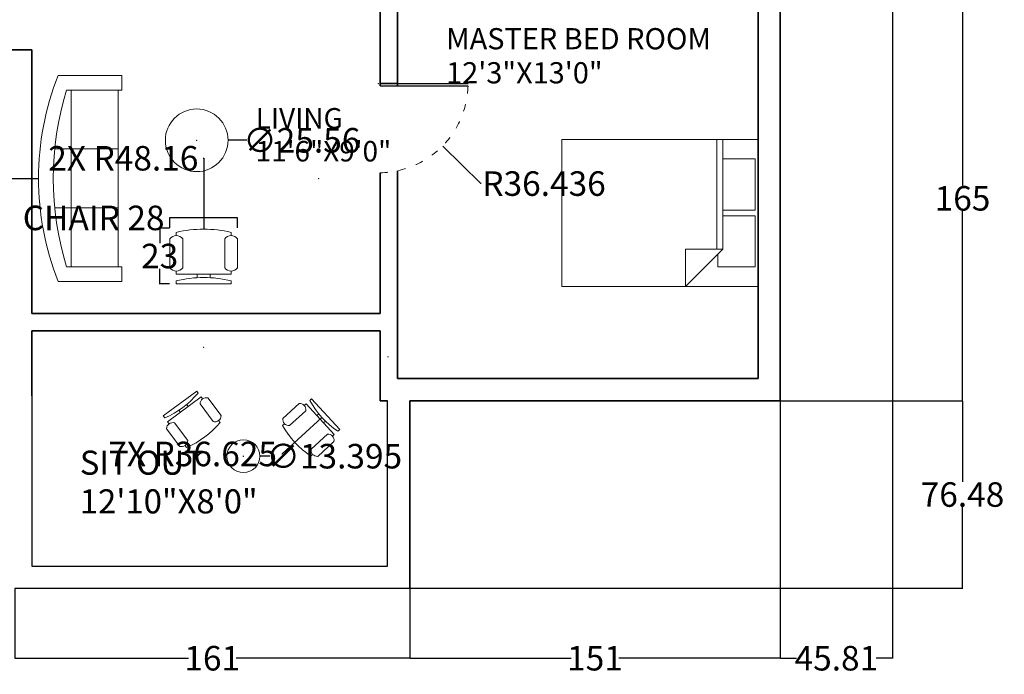
# Model space of a CAD drawing. Units: inches. Extents: x 37 to 687, y -399 to 163.
# Tile 2 of 4: x 286 to 687, y -399 to -132. Entities that reach past the tile are written whole.
import ezdxf

# ---------------------------------------------------------------- set-up
doc = ezdxf.new("R2010")
doc.units = ezdxf.units.IN
doc.header["$MEASUREMENT"] = 0
doc.linetypes.add('ACAD_ISO03W100', pattern=[30, 12, -18])
for name, color, linetype, lineweight in [('A-ANNO-DIMS', 2, 'Continuous', 18), ('A-AREA-IDEN', 7, 'Continuous', 18), ('A-DOOR', 4, 'Continuous', 25), ('A-DOOR-SWNG', 4, 'ACAD_ISO03W100', 13), ('A-FLOR-OTLN', 7, 'Continuous', 25), ('A-FURN', 8, 'Continuous', 18), ('A-WALL', 7, 'Continuous', 35)]:
    doc.layers.add(name, color=color, linetype=linetype, lineweight=lineweight)
doc.styles.get("Standard").update_dxf_attribs({"font": 'arial.ttf'})
doc.dimstyles.get("Standard").update_dxf_attribs({"dimtxt": 10, "dimasz": 0.18, "dimexe": 0.18, "dimexo": 0.0625, "dimgap": 0.09, "dimtad": 0, "dimtih": 1, "dimtoh": 1, "dimdec": 0, "dimzin": 0, "dimdsep": 46, "dimlunit": 3, "dimtxsty": 'Standard', "dimcen": 0.09, "dimadec": 0, "dimazin": 0, "dimtfac": 1, "dimtdec": 0, "dimtofl": 0, "dimtmove": 0, "dimatfit": 3, "dimfxl": 1, "dimtolj": 1, "dimtzin": 0, "dimarcsym": 0})

# ---------------------------------------------------------------- blocks, each defined once
blk = doc.blocks.new('Bed - Queen')
for p, q in [((0, -80.00003), (0, 0)), ((0, 0), (59.99999, 0)), ((59.99999, 0), (59.99999, -80.00003)), ((7.99999, -1.2), (28.79998, -1.2)), ((7.99999, -14.4), (7.99999, -1.2)), ((28.79998, -1.2), (28.79998, -14.4)), ((31.19999, -1.2), (51.99999, -1.2)), ((31.19999, -14.4), (31.19999, -1.2)), ((51.99999, -1.2), (51.99999, -16.4)), ((0, -14.4), (44.8, -14.4)), ((59.99999, -29.6), (44.8, -14.4)), ((44.8, -14.4), (44.8, -29.6)), ((44.8, -16.8), (0, -16.8)), ((51.99999, -16.4), (46.79936, -16.4)), ((44.8, -29.6), (59.99999, -29.6)), ((59.99999, -80.00003), (0, -80.00003))]:
    blk.add_line(p, q)
blk = doc.blocks.new('Chair - Desk')
for p, q in [((-8.5, 0), (-8.5, -1)), ((-8.5, 0), (8.5, 0)), ((8.5, 0), (8.5, -1)), ((-8.5, -3), (-8.5, -4)), ((-8.5, -3), (8.5, -3)), ((-2, -3), (-2, -1.9355)), ((2, -1.9576), (2, -3)), ((8.5, -3), (8.5, -4)), ((-10.5, -5), (-10.5, -14)), ((-6.5, -14), (-6.5, -5)), ((6.5, -5), (6.5, -14)), ((10.5, -14), (10.5, -5)), ((-8.5, -15), (-8.5, -16)), ((8.5, -15), (8.5, -16))]:
    blk.add_line(p, q)
for centre, radius, start, end in [((0, 34.625), 36.625, 256.5803, 283.4197), ((-8.5, -6.5), 2.5, 36.8699, 143.1301), ((8.5, -6.5), 2.5, 36.8699, 143.1301), ((-8.5, -12.5), 2.5, 216.8699, 323.1301), ((8.5, -12.5), 2.5, 216.8699, 323.1301), ((0, 19.625), 36.625, 256.5803, 283.4197)]:
    blk.add_arc(centre, radius, start, end)
blk = doc.blocks.new('Sofa - Roundback 7 ft.')
for p, q in [((-12.00002, -32.4421), (-12.00003, -6.5971)), ((11.99997, -32.4421), (11.99998, -6.5971)), ((-36.000027, -34), (-36.000027, -11.4696)), ((35.99998, -34), (35.99998, -11.4696)), ((-35.999844, -13.3819), (35.9998, -13.3819)), ((-36.000027, -32.4421), (35.99998, -32.4421))]:
    blk.add_line(p, q)
for points in [[(-36.000027, -34), (-42.000027, -34), (-42.000027, -8)], [(41.99998, -8), (41.99998, -34), (35.99998, -34)]]:
    blk.add_lwpolyline(points)
for centre, radius, start, end in [((0, -114.25), 114.25, 68.43141, 111.5686), ((-0.00001, -127.1968), 121.1968, 72.72033, 107.2797)]:
    blk.add_arc(centre, radius, start, end)
blk = doc.blocks.new('*D13')
at = {"layer": 'A-ANNO-DIMS', "color": 0, "lineweight": -2, "ltscale": 0.25, "transparency": 16777216}
for p, q in [((346.91, -213.16), (346.73, -213.16)), ((346.91, -217.24), (346.91, -212.98)), ((374.34, -213.16), (347.09, -213.16)), ((374.52, -217.24), (374.52, -212.98))]:
    blk.add_line(p, q, dxfattribs=at)
at = {"layer": 'A-ANNO-DIMS', "color": 0, "ltscale": 0.25, "transparency": 16777216}
for points in [[(347.09, -213.13), (347.09, -213.19), (346.91, -213.16)], [(374.34, -213.13), (374.34, -213.19), (374.52, -213.16)]]:
    blk.add_solid(points, dxfattribs=at)
at = {"layer": 'Defpoints', "color": 0, "ltscale": 0.25, "transparency": 16777216}
for p in [(346.91, -213.16), (346.91, -217.3), (374.52, -217.3)]:
    blk.add_point(p, dxfattribs=at)
at = {"layer": 'A-ANNO-DIMS', "color": 0, "ltscale": 0.25, "transparency": 16777216, "insert": (315.85, -213.16), "char_height": 10, "attachment_point": 5}
blk.add_mtext('\\A1;CHAIR 28', dxfattribs=at)
blk = doc.blocks.new('*D14')
at = {"layer": 'A-ANNO-DIMS', "color": 0, "lineweight": -2, "ltscale": 0.25, "transparency": 16777216}
for p, q in [((346.84, -217.3), (342.59, -217.3)), ((342.77, -217.48), (342.77, -223.5)), ((342.77, -239.92), (342.77, -233.9)), ((346.84, -240.1), (342.59, -240.1))]:
    blk.add_line(p, q, dxfattribs=at)
at = {"layer": 'A-ANNO-DIMS', "color": 0, "ltscale": 0.25, "transparency": 16777216}
for points in [[(342.74, -217.48), (342.8, -217.48), (342.77, -217.3)], [(342.74, -239.92), (342.8, -239.92), (342.77, -240.1)]]:
    blk.add_solid(points, dxfattribs=at)
at = {"layer": 'Defpoints', "color": 0, "ltscale": 0.25, "transparency": 16777216}
for p in [(346.91, -217.3), (342.77, -240.1), (346.91, -240.1)]:
    blk.add_point(p, dxfattribs=at)
at = {"layer": 'A-ANNO-DIMS', "color": 0, "ltscale": 0.25, "transparency": 16777216, "insert": (342.77, -228.7), "char_height": 10, "attachment_point": 5}
blk.add_mtext('\\A1;23', dxfattribs=at)
blk = doc.blocks.new('*D31')
at = {"layer": 'A-ANNO-DIMS', "color": 0, "lineweight": -2, "ltscale": 0.25, "transparency": 16777216}
for p, q in [((283.69, -364.23), (283.69, -392.85)), ((444.69, -364.23), (444.69, -392.85)), ((283.87, -392.67), (354.48, -392.67)), ((444.51, -392.67), (373.89, -392.67))]:
    blk.add_line(p, q, dxfattribs=at)
at = {"layer": 'A-ANNO-DIMS', "color": 0, "ltscale": 0.25, "transparency": 16777216}
for points in [[(283.87, -392.64), (283.87, -392.7), (283.69, -392.67)], [(444.51, -392.64), (444.51, -392.7), (444.69, -392.67)]]:
    blk.add_solid(points, dxfattribs=at)
at = {"layer": 'Defpoints', "color": 0, "ltscale": 0.25, "transparency": 16777216}
for p in [(283.69, -364.17), (444.69, -364.17), (444.69, -392.67)]:
    blk.add_point(p, dxfattribs=at)
at = {"layer": 'A-ANNO-DIMS', "color": 0, "ltscale": 0.25, "transparency": 16777216, "insert": (364.19, -392.67), "char_height": 10, "attachment_point": 5}
blk.add_mtext('\\A1;161', dxfattribs=at)
blk = doc.blocks.new('*D32')
at = {"layer": 'A-ANNO-DIMS', "color": 0, "lineweight": -2, "ltscale": 0.25, "transparency": 16777216}
for p, q in [((444.69, -287.75), (444.69, -392.85)), ((595.69, -287.75), (595.69, -392.85)), ((444.87, -392.67), (510.48, -392.67)), ((595.51, -392.67), (529.89, -392.67))]:
    blk.add_line(p, q, dxfattribs=at)
at = {"layer": 'A-ANNO-DIMS', "color": 0, "ltscale": 0.25, "transparency": 16777216}
for points in [[(444.87, -392.64), (444.87, -392.7), (444.69, -392.67)], [(595.51, -392.64), (595.51, -392.7), (595.69, -392.67)]]:
    blk.add_solid(points, dxfattribs=at)
at = {"layer": 'Defpoints', "color": 0, "ltscale": 0.25, "transparency": 16777216}
for p in [(444.69, -287.68), (595.69, -287.68), (595.69, -392.67)]:
    blk.add_point(p, dxfattribs=at)
at = {"layer": 'A-ANNO-DIMS', "color": 0, "ltscale": 0.25, "transparency": 16777216, "insert": (520.19, -392.67), "char_height": 10, "attachment_point": 5}
blk.add_mtext('\\A1;151', dxfattribs=at)
blk = doc.blocks.new('*D33')
at = {"layer": 'A-ANNO-DIMS', "color": 0, "lineweight": -2, "ltscale": 0.25, "transparency": 16777216}
for p, q in [((641.5, -122.75), (641.5, -392.85)), ((595.69, -287.75), (595.69, -392.85)), ((595.87, -392.67), (602.39, -392.67)), ((641.32, -392.67), (634.79, -392.67))]:
    blk.add_line(p, q, dxfattribs=at)
at = {"layer": 'A-ANNO-DIMS', "color": 0, "ltscale": 0.25, "transparency": 16777216}
for points in [[(595.87, -392.64), (595.87, -392.7), (595.69, -392.67)], [(641.32, -392.64), (641.32, -392.7), (641.5, -392.67)]]:
    blk.add_solid(points, dxfattribs=at)
at = {"layer": 'Defpoints', "color": 0, "ltscale": 0.25, "transparency": 16777216}
for p in [(641.5, -122.68), (595.69, -287.68), (641.5, -392.67)]:
    blk.add_point(p, dxfattribs=at)
at = {"layer": 'A-ANNO-DIMS', "color": 0, "ltscale": 0.25, "transparency": 16777216, "insert": (618.59, -392.67), "char_height": 10, "attachment_point": 5}
blk.add_mtext('\\A1;45.81', dxfattribs=at)
blk = doc.blocks.new('*D36')
at = {"layer": 'A-ANNO-DIMS', "color": 0, "lineweight": -2, "ltscale": 0.25, "transparency": 16777216}
for p, q in [((595.75, -122.68), (670.18, -122.68)), ((670, -122.86), (670, -199.99)), ((670, -287.5), (670, -210.38)), ((595.75, -287.68), (670.18, -287.68))]:
    blk.add_line(p, q, dxfattribs=at)
at = {"layer": 'A-ANNO-DIMS', "color": 0, "ltscale": 0.25, "transparency": 16777216}
for points in [[(669.97, -122.86), (670.03, -122.86), (670, -122.68)], [(669.97, -287.5), (670.03, -287.5), (670, -287.68)]]:
    blk.add_solid(points, dxfattribs=at)
at = {"layer": 'Defpoints', "color": 0, "ltscale": 0.25, "transparency": 16777216}
for p in [(595.69, -122.68), (670, -122.68), (595.69, -287.68)]:
    blk.add_point(p, dxfattribs=at)
at = {"layer": 'A-ANNO-DIMS', "color": 0, "ltscale": 0.25, "transparency": 16777216, "insert": (670, -205.18), "char_height": 10, "attachment_point": 5}
blk.add_mtext('\\A1;165', dxfattribs=at)
blk = doc.blocks.new('*D37')
at = {"layer": 'A-ANNO-DIMS', "color": 0, "lineweight": -2, "ltscale": 0.25, "transparency": 16777216}
for p, q in [((595.75, -287.68), (670.18, -287.68)), ((670, -287.86), (670, -320.73)), ((670, -363.99), (670, -331.12)), ((444.75, -364.17), (670.18, -364.17))]:
    blk.add_line(p, q, dxfattribs=at)
at = {"layer": 'A-ANNO-DIMS', "color": 0, "ltscale": 0.25, "transparency": 16777216}
for points in [[(669.97, -287.86), (670.03, -287.86), (670, -287.68)], [(669.97, -363.99), (670.03, -363.99), (670, -364.17)]]:
    blk.add_solid(points, dxfattribs=at)
at = {"layer": 'Defpoints', "color": 0, "ltscale": 0.25, "transparency": 16777216}
for p in [(595.69, -287.68), (670, -287.68), (444.69, -364.17)]:
    blk.add_point(p, dxfattribs=at)
at = {"layer": 'A-ANNO-DIMS', "color": 0, "ltscale": 0.25, "transparency": 16777216, "insert": (670, -325.93), "char_height": 10, "attachment_point": 5}
blk.add_mtext('\\A1;76.48', dxfattribs=at)
blk = doc.blocks.new('*D46')
at = {"layer": 'A-ANNO-DIMS', "color": 0, "lineweight": -2, "ltscale": 0.25, "transparency": 16777216}
for p, q in [((357.77, -181.52), (357.95, -181.52)), ((357.86, -181.61), (357.86, -181.43)), ((378.31, -181.52), (370.82, -181.52))]:
    blk.add_line(p, q, dxfattribs=at)
at = {"layer": 'A-ANNO-DIMS', "color": 0, "ltscale": 0.25, "transparency": 16777216}
blk.add_solid([(370.82, -181.49), (370.82, -181.55), (370.64, -181.52)], dxfattribs=at)
at = {"layer": 'Defpoints', "color": 0, "ltscale": 0.25, "transparency": 16777216}
for p in [(345.08, -181.52), (370.64, -181.52)]:
    blk.add_point(p, dxfattribs=at)
at = {"layer": 'A-ANNO-DIMS', "color": 0, "ltscale": 0.25, "transparency": 16777216, "insert": (400.71, -181.52), "char_height": 10, "attachment_point": 5}
blk.add_mtext('\\A1;∅25.56', dxfattribs=at)
blk = doc.blocks.new('*D47')
at = {"layer": 'A-ANNO-DIMS', "color": 0, "lineweight": -2, "ltscale": 0.25, "transparency": 16777216}
for p, q in [((376.8, -310.3), (376.98, -310.3)), ((376.89, -310.39), (376.89, -310.21)), ((387.61, -310.3), (383.77, -310.3))]:
    blk.add_line(p, q, dxfattribs=at)
at = {"layer": 'A-ANNO-DIMS', "color": 0, "ltscale": 0.25, "transparency": 16777216}
blk.add_solid([(383.77, -310.27), (383.77, -310.33), (383.59, -310.3)], dxfattribs=at)
at = {"layer": 'Defpoints', "color": 0, "ltscale": 0.25, "transparency": 16777216}
for p in [(370.2, -310.3), (383.59, -310.3)]:
    blk.add_point(p, dxfattribs=at)
at = {"layer": 'A-ANNO-DIMS', "color": 0, "ltscale": 0.25, "transparency": 16777216, "insert": (413.93, -310.3), "char_height": 10, "attachment_point": 5}
blk.add_mtext('\\A1;∅13.395', dxfattribs=at)
blk = doc.blocks.new('*D50')
at = {"layer": 'A-ANNO-DIMS', "color": 0, "lineweight": -2, "ltscale": 0.25, "transparency": 16777216}
for p, q in [((431.94, -158.31), (432.12, -158.31)), ((432.03, -158.4), (432.03, -158.22)), ((473.62, -199.16), (458.15, -183.97)), ((473.8, -199.16), (473.62, -199.16))]:
    blk.add_line(p, q, dxfattribs=at)
at = {"layer": 'A-ANNO-DIMS', "color": 0, "ltscale": 0.25, "transparency": 16777216}
blk.add_solid([(458.18, -183.95), (458.13, -183.99), (458.03, -183.84)], dxfattribs=at)
at = {"layer": 'Defpoints', "color": 0, "ltscale": 0.25, "transparency": 16777216}
for p in [(432.03, -158.31), (458.03, -183.84)]:
    blk.add_point(p, dxfattribs=at)
at = {"layer": 'A-ANNO-DIMS', "color": 0, "ltscale": 0.25, "transparency": 16777216, "insert": (499.43, -199.16), "char_height": 10, "attachment_point": 5}
blk.add_mtext('\\A1;R36.436', dxfattribs=at)
blk = doc.blocks.new('*D55')
at = {"layer": 'A-ANNO-DIMS', "color": 0, "lineweight": -2, "ltscale": 0.25, "transparency": 16777216}
for p, q in [((224.82, -197.06), (293.19, -197.06)), ((407.53, -197.06), (407.71, -197.06)), ((407.62, -197.15), (407.62, -196.97))]:
    blk.add_line(p, q, dxfattribs=at)
at = {"layer": 'A-ANNO-DIMS', "color": 0, "ltscale": 0.25, "transparency": 16777216}
blk.add_solid([(293.19, -197.03), (293.19, -197.09), (293.37, -197.06)], dxfattribs=at)
at = {"layer": 'Defpoints', "color": 0, "ltscale": 0.25, "transparency": 16777216}
for p in [(293.37, -197.06), (407.62, -197.06)]:
    blk.add_point(p, dxfattribs=at)
at = {"layer": 'A-ANNO-DIMS', "color": 0, "ltscale": 0.25, "transparency": 16777216, "insert": (188.33, -197.06), "char_height": 10, "attachment_point": 5}
blk.add_mtext('\\A1;2X R114.25', dxfattribs=at)
blk = doc.blocks.new('*D56')
at = {"layer": 'A-ANNO-DIMS', "color": 0, "lineweight": -2, "ltscale": 0.25, "transparency": 16777216}
for p, q in [((360.53, -188.84), (360.71, -188.84)), ((360.71, -188.84), (360.71, -217.56)), ((360.63, -265.9), (360.81, -265.9)), ((360.72, -265.99), (360.72, -265.81))]:
    blk.add_line(p, q, dxfattribs=at)
at = {"layer": 'A-ANNO-DIMS', "color": 0, "ltscale": 0.25, "transparency": 16777216}
blk.add_solid([(360.74, -217.56), (360.68, -217.56), (360.71, -217.74)], dxfattribs=at)
at = {"layer": 'Defpoints', "color": 0, "ltscale": 0.25, "transparency": 16777216}
for p in [(360.71, -217.74), (360.72, -265.9)]:
    blk.add_point(p, dxfattribs=at)
at = {"layer": 'A-ANNO-DIMS', "color": 0, "ltscale": 0.25, "transparency": 16777216, "insert": (327.96, -188.84), "char_height": 10, "attachment_point": 5}
blk.add_mtext('\\A1;2X R48.16', dxfattribs=at)
blk = doc.blocks.new('*D57')
at = {"layer": 'A-ANNO-DIMS', "color": 0, "lineweight": -2, "ltscale": 0.25, "transparency": 16777216}
for p, q in [((435.79, -269.73), (435.97, -269.73)), ((435.88, -269.82), (435.88, -269.64)), ((392.75, -309.39), (408.79, -294.64)), ((392.57, -309.39), (392.75, -309.39))]:
    blk.add_line(p, q, dxfattribs=at)
at = {"layer": 'A-ANNO-DIMS', "color": 0, "ltscale": 0.25, "transparency": 16777216}
blk.add_solid([(408.77, -294.62), (408.81, -294.66), (408.92, -294.52)], dxfattribs=at)
at = {"layer": 'Defpoints', "color": 0, "ltscale": 0.25, "transparency": 16777216}
for p in [(435.88, -269.73), (408.92, -294.52)]:
    blk.add_point(p, dxfattribs=at)
at = {"layer": 'A-ANNO-DIMS', "color": 0, "ltscale": 0.25, "transparency": 16777216, "insert": (356.2, -309.39), "char_height": 10, "attachment_point": 5}
blk.add_mtext('\\A1;7X R36.625', dxfattribs=at)

msp = doc.modelspace()

# ---------------------------------------------------------------- linework, layer by layer
at = {"layer": 'A-DOOR', "ltscale": 0.25}
for p, q in [((432.6852, -158.3108), (468.4684, -158.3108)), ((432.6852, -158.3108), (432.6852, -159.3108)), ((432.6852, -159.3108), (468.4684, -159.3108))]:
    msp.add_line(p, q, dxfattribs=at)
at = {"layer": 'A-DOOR-SWNG', "ltscale": 0.25}
msp.add_arc((432.0327, -158.3108), 36.4357, 271.026022, 0, dxfattribs=at)
at = {"layer": 'A-FLOR-OTLN'}
for p, q in [((290.6852, -259.1681), (290.6852, -355.1681)), ((435.6852, -355.1681), (435.6852, -287.6846)), ((444.6852, -364.1681), (444.6852, -287.6846)), ((290.6852, -355.1681), (435.6852, -355.1681)), ((283.6852, -364.1681), (444.6852, -364.1681))]:
    msp.add_line(p, q, dxfattribs=at)
at = {"layer": 'A-FURN', "ltscale": 0.25}
for centre, radius in [((357.863, -181.5218), 12.7799), ((376.8936, -310.3015), 6.6973)]:
    msp.add_circle(centre, radius, dxfattribs=at)
at = {"layer": 'A-WALL'}
for p, q in [((432.6852, -159.3108), (432.6852, -113.6846)), ((439.6852, -159.3108), (439.6852, -122.6846)), ((586.6852, -122.6846), (586.6852, -278.6846)), ((595.6852, -122.6846), (595.6852, -278.6846)), ((595.6852, -122.6846), (595.6852, -287.6846)), ((290.6852, -144.6846), (282.6852, -144.6846)), ((290.6852, -252.1681), (290.6852, -144.6846)), ((432.6852, -252.1681), (432.6852, -194.7406)), ((439.6852, -278.6846), (439.6852, -193.9338)), ((290.6852, -252.1681), (432.6852, -252.1681)), ((290.6852, -285.6846), (290.6852, -259.1681)), ((290.6852, -259.1681), (432.6852, -259.1681)), ((432.6852, -287.6846), (432.6852, -259.1681)), ((586.6852, -278.6846), (439.6852, -278.6846)), ((435.6852, -287.6846), (432.6852, -287.6846)), ((595.6852, -287.6846), (444.6852, -287.6846))]:
    msp.add_line(p, q, dxfattribs=at)
at = {"layer": 'A-WALL', "ltscale": 0.25}
msp.add_line((432.6852, -158.3108), (439.6852, -158.3108), dxfattribs=at)

# ---------------------------------------------------------------- block references
at = {"layer": 'A-FURN', "ltscale": 0.25}
for name, p, rotation in [('Sofa - Roundback 7 ft.', (293.3737, -197.0564), 90), ('Bed - Queen', (586.6852, -181.1397), 270), ('Chair - Desk', (351.0371, -288.8154), 36.65650432641661), ('Chair - Desk', (410.3969, -293.163), 312.6021142339054)]:
    msp.add_blockref(name, p, dxfattribs=dict(at, rotation=rotation))
at = {"layer": 'A-FURN', "ltscale": 0.25, "xscale": 1.315011609318839, "yscale": 1.315011609318839, "zscale": 1.315011609318839, "rotation": 180}
msp.add_blockref('Chair - Desk', (360.7151, -240.096), dxfattribs=at)

# ---------------------------------------------------------------- texts
at = {"layer": 'A-AREA-IDEN', "ltscale": 0.25}
for s, height, p in [('MASTER BED ROOM', 8.643392, (459.5422, -144.426)), ('12\'3"X13\'0"', 8.643392, (459.5422, -158.3108)), ('LIVING ', 8.35031, (381.9042, -176.7313)), ('11\'6"X9\'0"', 8.35031, (381.9042, -190.1453)), ('SIT OUT ', 9.82505, (310.2196, -317.8501)), ('12\'10"X8\'0"', 9.825048, (310.2196, -333.6332))]:
    msp.add_text(s, height=height, dxfattribs=at).set_placement(p)

# ---------------------------------------------------------------- dimensions: what is measured, and where the dimension line sits
at = {"layer": 'A-ANNO-DIMS', "ltscale": 0.25}
for base, p1, p2, override, picture, middle in [((641.4983, -392.6681), (595.6852, -287.6846), (641.4983, -122.6846), {"dimdec": 2, "dimlfac": 1, "dimrnd": 0, "dimzin": 0, "dimdsep": 46, "dimlunit": 2}, '*D33', (618.5917, -392.6681)), ((595.6852, -392.6681), (444.6852, -287.6846), (595.6852, -287.6846), {"dimdec": 0, "dimlfac": 1, "dimrnd": 0, "dimzin": 0, "dimdsep": 46, "dimlunit": 2}, '*D32', (520.1852, -392.6681)), ((444.6852, -392.6681), (283.6852, -364.1681), (444.6852, -364.1681), {"dimdec": 0, "dimlfac": 1, "dimrnd": 0, "dimzin": 0, "dimdsep": 46, "dimlunit": 2}, '*D31', (364.1852, -392.6681))]:
    dim = msp.add_linear_dim(base=base, p1=p1, p2=p2, dimstyle='Standard', override=override, dxfattribs=at)
    dim.commit()
    dim.dimension.update_dxf_attribs({"geometry": picture, "text_midpoint": middle})
for base, p1, p2, angle, override, picture, middle in [((669.9983, -122.6846), (595.6852, -287.6846), (595.6852, -122.6846), 90, {"dimdec": 0, "dimlfac": 1, "dimrnd": 0, "dimzin": 0, "dimdsep": 46, "dimlunit": 2}, '*D36', (669.9983, -205.1846)), ((342.7652, -240.096), (346.9075, -217.3025), (346.9075, -240.096), 270, {"dimdec": 0, "dimlfac": 1, "dimrnd": 0, "dimzin": 0, "dimdsep": 46, "dimlunit": 2}, '*D14', (342.7652, -228.6993)), ((669.9983, -287.6846), (444.6852, -364.1681), (595.6852, -287.6846), 90, {"dimdec": 2, "dimlfac": 1, "dimrnd": 0, "dimzin": 0, "dimdsep": 46, "dimlunit": 2}, '*D37', (669.9983, -325.9263))]:
    dim = msp.add_linear_dim(base=base, p1=p1, p2=p2, angle=angle, dimstyle='Standard', override=override, dxfattribs=at)
    dim.commit()
    dim.dimension.update_dxf_attribs({"geometry": picture, "text_midpoint": middle})
dim = msp.add_radius_dim(center=(432.0327, -158.3108), mpoint=(458.0262, -183.8432), dimstyle='Standard', override={"dimdec": 3, "dimlfac": 1, "dimrnd": 0, "dimzin": 0, "dimdsep": 46, "dimlunit": 2}, dxfattribs=at)
dim.commit()
dim.dimension.update_dxf_attribs({"geometry": '*D50', "text_midpoint": (499.4311, -199.1626), "dimtype": 164})
for center, mpoint, text, override, picture, middle in [((360.7151, -265.9031), (360.715, -217.7408), '2X <>', {"dimdec": 2, "dimlfac": 1, "dimrnd": 0, "dimzin": 0, "dimdsep": 46, "dimlunit": 2}, '*D56', (327.962, -188.8435)), ((407.6237, -197.0564), (293.3737, -197.056), '2X <>', {"dimdec": 2, "dimlfac": 1, "dimrnd": 0, "dimzin": 0, "dimdsep": 46, "dimlunit": 2}, '*D55', (224.8237, -197.0557)), ((435.8834, -269.7252), (408.9249, -294.5171), '7X <>', {"dimdec": 3, "dimlfac": 1, "dimrnd": 0, "dimzin": 0, "dimdsep": 46, "dimlunit": 2}, '*D57', (356.1975, -309.3921))]:
    dim = msp.add_radius_dim(center=center, mpoint=mpoint, text=text, dimstyle='Standard', override=override, dxfattribs=at)
    dim.commit()
    dim.dimension.update_dxf_attribs({"geometry": picture, "text_midpoint": middle, "dimtype": 164})
for p1, p2, override, picture, middle in [((345.0831, -181.5216), (370.6429, -181.522), {"dimdec": 2, "dimlfac": 1, "dimrnd": 0, "dimzin": 0, "dimdsep": 46, "dimlunit": 2}, '*D46', (378.3108, -181.5221)), ((370.1963, -310.302), (383.5909, -310.301), {"dimdec": 3, "dimlfac": 1, "dimrnd": 0, "dimzin": 0, "dimdsep": 46, "dimlunit": 2}, '*D47', (387.6092, -310.3007))]:
    dim = msp.add_diameter_dim_2p(p1=p1, p2=p2, dimstyle='Standard', override=override, dxfattribs=at)
    dim.commit()
    dim.dimension.update_dxf_attribs({"geometry": picture, "text_midpoint": middle, "dimtype": 163})
dim = msp.add_linear_dim(base=(346.9075, -213.1602), p1=(374.5227, -217.3025), p2=(346.9075, -217.3025), angle=180, text='CHAIR <>', dimstyle='Standard', override={"dimdec": 0, "dimlfac": 1, "dimrnd": 0, "dimzin": 0, "dimdsep": 46, "dimlunit": 2}, dxfattribs=at)
dim.commit()
dim.dimension.update_dxf_attribs({"geometry": '*D13', "text_midpoint": (315.8496, -213.1602)})

doc.saveas('drawing.dxf')
